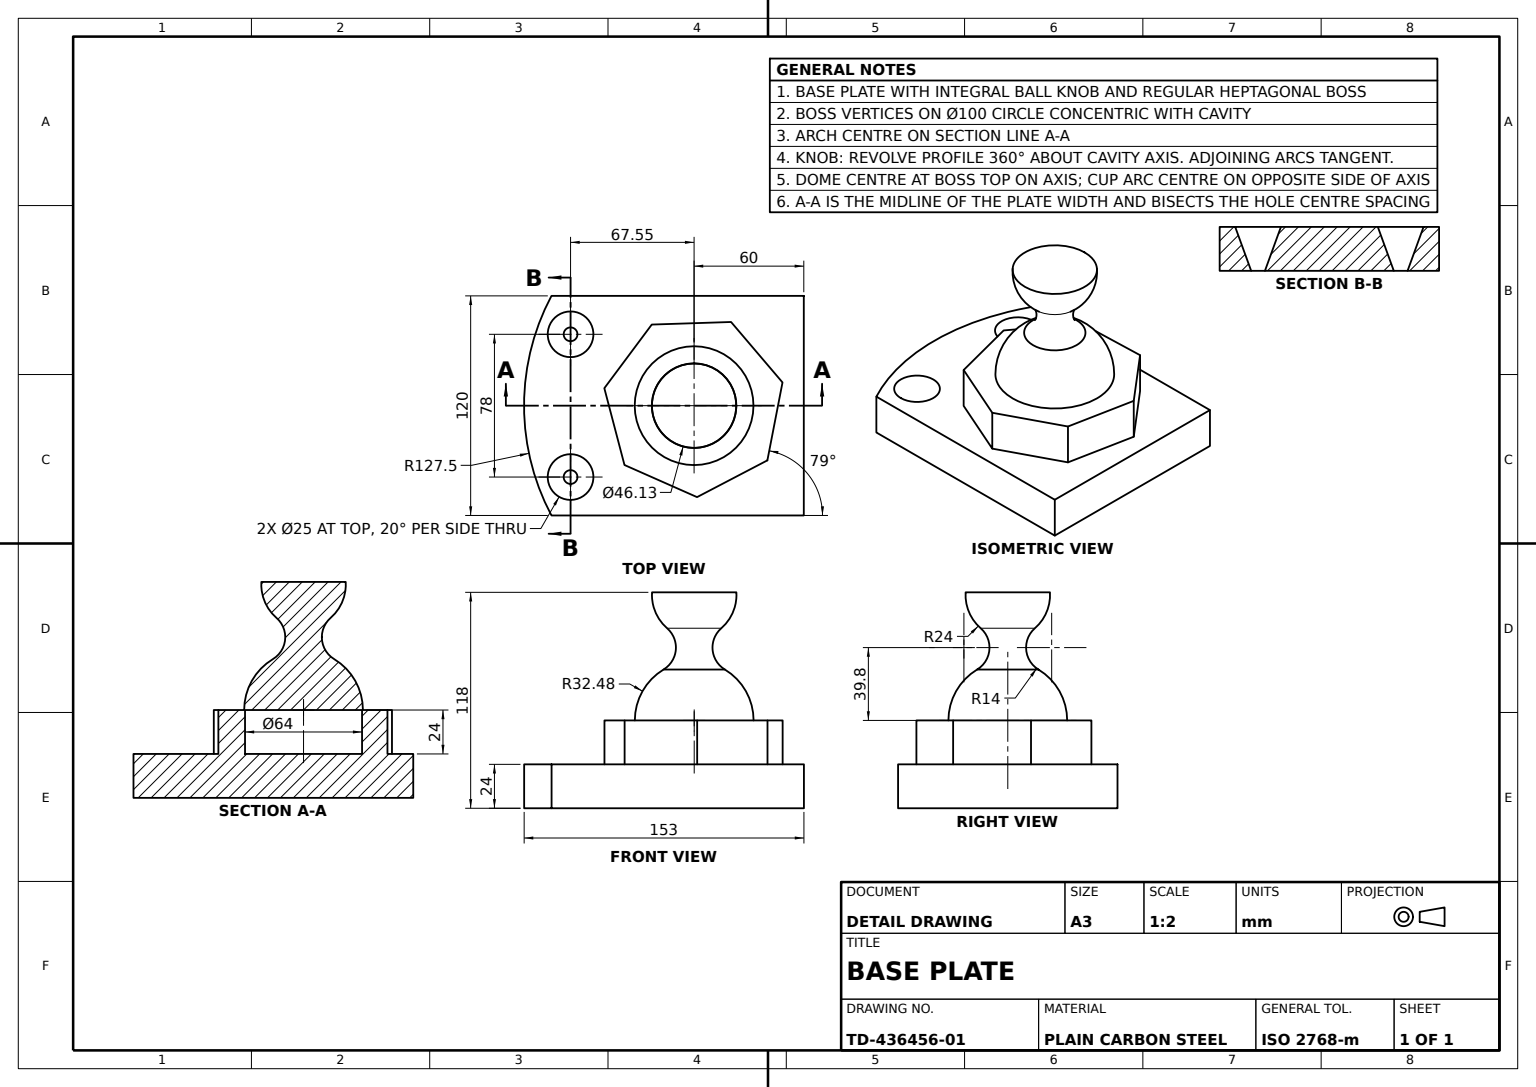
SolidWorks part; units mm, degrees
material "Plain Carbon Steel"
ref_plane "Front Plane" through (0, 0, 0) normal (0, 0, 1) x (1, 0, 0)
ref_plane "Top Plane" through (0, 0, 0) normal (0, 1, 0) x (1, 0, 0)
ref_plane "Right Plane" through (0, 0, 0) normal (1, 0, 0) x (0, 0, -1)
sketch "Knob Profile Sketch" plane through (0, 0, 0) normal (0, 0, 1) x (1, 0, 0)
  line L0 (0, 0) -> (0, 70)
  line L1 (0, 70) -> (23.065, 70)
  line L2 (0, 0) -> (32.4762, 0)
  arc A0 (14.8304, 50.3791) -> (16.7705, 27.8111) centre (24, 39.8) ccw
  arc A1 (14.8304, 50.3791) -> (23.065, 70) centre (-0.889, 68.5148) ccw
  arc A2 (32.4762, 0) -> (16.7705, 27.8111) centre (0, 0) ccw
  dimension "D2" = 28
  dimension "D4" = 24
  dimension "D5" = 23.065
  dimension "D6" = 70
  dimension "D1" = 39.8
  dimension "D3" = 24
revolve "Ball Knob" add sketch "Knob Profile Sketch" angle 360 about L0
sketch "Hex Boss Sketch" plane through (0, 0, 0) normal (0, -1, 0) x (1, 0, 0)
  line L1 (1.6198, 49.9738) -> (-38.0611, 32.4246)
  line L2 (-38.0611, 32.4246) -> (-49.0813, -9.541)
  line L3 (-49.0813, -9.541) -> (-23.1422, -44.322)
  line L4 (-23.1422, -44.322) -> (20.2234, -45.7276)
  line L5 (20.2234, -45.7276) -> (48.3604, -12.6994)
  line L6 (48.3604, -12.6994) -> (40.081, 29.8917)
  line L7 (40.081, 29.8917) -> (1.6198, 49.9738)
  circle A0 centre (0, 0) radius 50 construction
  circle A1 centre (0, 0) radius 45.0484 construction
  circle A2 centre (0, 0) radius 32
  circle A3 centre (0, 0) radius 32.4762 construction
  dimension "D1" = 100
  dimension "D2" = 64
  dimension "D3" = 1.6198
extrude "Hex Boss" add sketch "Hex Boss Sketch" along normal blind 24
sketch "Base Plate Sketch" plane through (0, -24, 0) normal (0, -1, 0) x (1, 0, 0)
  line L0 (-78, 60) -> (60, 60)
  line L1 (60, 60) -> (60, -60)
  line L2 (60, -60) -> (-78, -60)
  arc A4 (-78, -60) -> (-78, 60) centre (34.5, 0) cw
  dimension "D4" = 127.5
  dimension "D5" = 138
  dimension "D1" = 120
  dimension "D2" = 60
  dimension "D3" = 60
  dimension "D6" = 138
extrude "Base Plate" add sketch "Base Plate Sketch" along normal blind 24
sketch "Plate Holes Sketch" plane through (0, -24, 0) normal (0, 1, 0) x (1, 0, 0)
  circle A0 centre (-67.55, 39) radius 12.5
  circle A1 centre (-67.55, -39) radius 12.5
  dimension "D1" = 25
  dimension "D2" = 25
  dimension "D3" = 78
  dimension "D4" = 67.55
  dimension "D5" = 39
extrude "Plate Holes 2xØ25" cut sketch "Plate Holes Sketch" against normal up to surface (24 mm away) draft 20 up to face at (-12.75, -48, 0)
